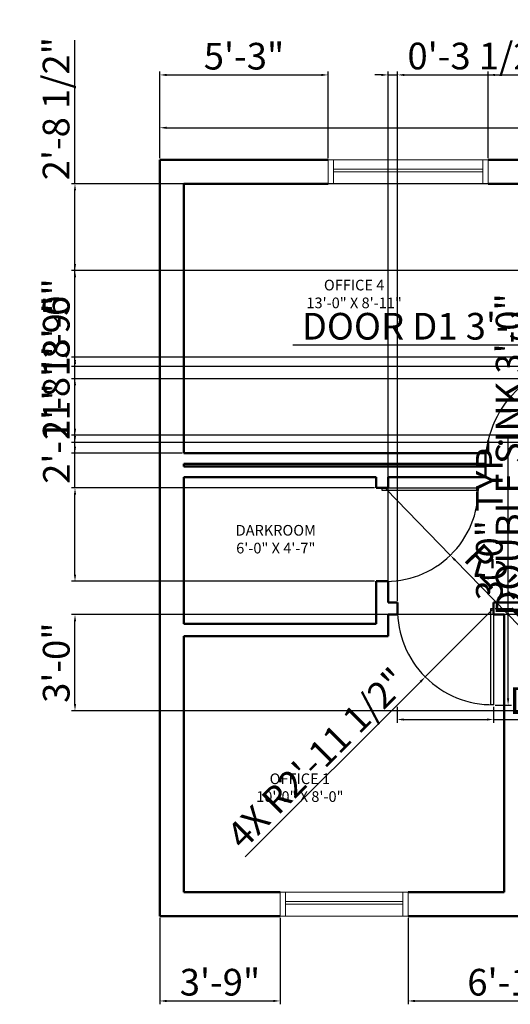
# Model space of a CAD drawing. Units: inches. Extents: x -53 to 650, y -41 to 348.
# Tile 1 of 3: x -53 to 131, y -33 to 336. Entities that reach past the tile are written whole.
import ezdxf

# ---------------------------------------------------------------- set-up
doc = ezdxf.new("R2010")
doc.units = ezdxf.units.IN
for name, color, linetype, lineweight in [('A-ANNO-DIMS', 2, 'Continuous', 18), ('A-AREA-IDEN', 7, 'Continuous', 25), ('A-DOOR', 3, 'Continuous', 25), ('A-GLAZ', 4, 'Continuous', 18), ('A-WALL', 7, 'Continuous', 50), ('A-WALL-PATT', 7, 'Continuous', 13)]:
    doc.layers.add(name, color=color, linetype=linetype, lineweight=lineweight)
doc.styles.get("Standard").update_dxf_attribs({"font": 'arial.ttf'})
doc.dimstyles.new('ISO-25', dxfattribs={"dimtxt": 10, "dimasz": 2.5, "dimexe": 1.25, "dimexo": 0.625, "dimtad": 1, "dimlunit": 4, "dimtxsty": 'Standard', "dimcen": 2.5, "dimadec": 0, "dimazin": 0, "dimtfac": 1, "dimtmove": 0, "dimatfit": 3, "dimfxl": 1, "dimarcsym": 0})

# ---------------------------------------------------------------- blocks, each defined once
blk = doc.blocks.new('*D4')
at = {"layer": 'A-ANNO-DIMS', "color": 0, "lineweight": -2, "transparency": 16777216}
for p, q in [((0, 284.12), (0, 296.76)), ((2.5, 295.51), (604.5, 295.51)), ((607, 284.12), (607, 296.76))]:
    blk.add_line(p, q, dxfattribs=at)
at = {"layer": 'A-ANNO-DIMS', "color": 0, "transparency": 16777216}
for points in [[(2.5, 295.92), (2.5, 295.09), (0, 295.51)], [(604.5, 295.92), (604.5, 295.09), (607, 295.51)]]:
    blk.add_solid(points, dxfattribs=at)
at = {"layer": 'Defpoints', "color": 0, "transparency": 16777216}
for p in [(607, 295.51), (0, 283.5), (607, 283.5)]:
    blk.add_point(p, dxfattribs=at)
at = {"layer": 'A-ANNO-DIMS', "color": 0, "transparency": 16777216, "insert": (303.5, 301.24), "char_height": 10, "attachment_point": 5}
blk.add_mtext('50\'-0"', dxfattribs=at)
blk = doc.blocks.new('DOOR-SWING-39IN')
for p, q in [((38, 0), (38, 39)), ((38, 39), (39, 39)), ((39, 39), (39, 0)), ((39, 0), (38, 0))]:
    blk.add_line(p, q)
blk.add_arc((38.5, 38.5), 38.5, 179.2559, 270.7441)
blk = doc.blocks.new('DOOR-SWING-36IN')
for p, q in [((35.001, 0.001), (35.001, 36.001)), ((35.001, 36.001), (36.001, 36.001)), ((36.001, 36.001), (36.001, 0.001)), ((36.001, 0.001), (35.001, 0.001))]:
    blk.add_line(p, q)
blk.add_arc((35.501, 35.501), 35.504, 179.19307, 270.80693)
blk = doc.blocks.new('WIN-48IN')
for p, q in [((0, 9), (0, 0)), ((2, 0), (2, 9)), ((46, 0), (46, 9)), ((48, 9), (48, 0)), ((2, 5.5), (46, 5.5)), ((2, 4.5), (46, 4.5))]:
    blk.add_line(p, q)
blk.add_lwpolyline([(48, 9), (0, 9), (0, 0), (48, 0)], close=True)
blk = doc.blocks.new('WIN-60IN')
for p, q in [((0, 9), (0, 0)), ((2, 0), (2, 9)), ((58, 0), (58, 9)), ((60, 9), (60, 0)), ((2, 5.5), (58, 5.5)), ((2, 4.5), (58, 4.5))]:
    blk.add_line(p, q)
blk.add_lwpolyline([(60, 9), (0, 9), (0, 0), (60, 0)], close=True)
blk = doc.blocks.new('*D11')
at = {"layer": 'A-ANNO-DIMS', "color": 0, "lineweight": -2, "transparency": 16777216}
for p, q in [((181.5, 208.76), (181.5, 215.26)), ((220.63, 208.76), (220.63, 215.26)), ((181.5, 214.01), (49.76, 214.01)), ((218.13, 214.01), (184, 214.01))]:
    blk.add_line(p, q, dxfattribs=at)
at = {"layer": 'A-ANNO-DIMS', "color": 0, "transparency": 16777216}
for points in [[(184, 214.42), (184, 213.59), (181.5, 214.01)], [(218.13, 214.42), (218.13, 213.59), (220.63, 214.01)]]:
    blk.add_solid(points, dxfattribs=at)
at = {"layer": 'Defpoints', "color": 0, "transparency": 16777216}
for p in [(181.5, 214.01), (181.5, 208.13), (220.63, 208.13)]:
    blk.add_point(p, dxfattribs=at)
at = {"layer": 'A-ANNO-DIMS', "color": 0, "transparency": 16777216, "insert": (114.38, 219.81), "char_height": 10, "attachment_point": 5}
blk.add_mtext('DOOR D1 3\'-3" TYP.', dxfattribs=at)
blk = doc.blocks.new('*D13')
at = {"layer": 'A-ANNO-DIMS', "color": 0, "lineweight": -2, "transparency": 16777216}
for p, q in [((88.86, 78.49), (88.86, 72.44)), ((125, 78.49), (125, 72.44)), ((91.36, 73.69), (122.5, 73.69)), ((125, 73.69), (256.74, 73.69))]:
    blk.add_line(p, q, dxfattribs=at)
at = {"layer": 'A-ANNO-DIMS', "color": 0, "transparency": 16777216}
for points in [[(91.36, 74.11), (91.36, 73.28), (88.86, 73.69)], [(122.5, 74.11), (122.5, 73.28), (125, 73.69)]]:
    blk.add_solid(points, dxfattribs=at)
at = {"layer": 'Defpoints', "color": 0, "transparency": 16777216}
for p in [(88.86, 79.11), (125, 79.11), (125, 73.69)]:
    blk.add_point(p, dxfattribs=at)
at = {"layer": 'A-ANNO-DIMS', "color": 0, "transparency": 16777216, "insert": (192.12, 79.5), "char_height": 10, "attachment_point": 5}
blk.add_mtext('DOOR D2 3\'-0" TYP.', dxfattribs=at)
blk = doc.blocks.new('*D14')
at = {"layer": 'A-ANNO-DIMS', "color": 0, "lineweight": -2, "transparency": 16777216}
for p, q in [((130.42, 115.25), (130.42, 179.95)), ((125.62, 115.25), (131.67, 115.25)), ((130.42, 81.61), (130.42, 112.75)), ((125.62, 79.11), (131.67, 79.11))]:
    blk.add_line(p, q, dxfattribs=at)
at = {"layer": 'A-ANNO-DIMS', "color": 0, "transparency": 16777216}
for points in [[(130, 112.75), (130.84, 112.75), (130.42, 115.25)], [(130, 81.61), (130.84, 81.61), (130.42, 79.11)]]:
    blk.add_solid(points, dxfattribs=at)
at = {"layer": 'Defpoints', "color": 0, "transparency": 16777216}
for p in [(125, 115.25), (130.42, 115.25), (125, 79.11)]:
    blk.add_point(p, dxfattribs=at)
at = {"layer": 'A-ANNO-DIMS', "color": 0, "transparency": 16777216, "insert": (124.69, 148.85), "char_height": 10, "attachment_point": 5, "rotation": 90}
blk.add_mtext('3\'-0" TYP.', dxfattribs=at)
blk = doc.blocks.new('*D21')
at = {"layer": 'A-ANNO-DIMS', "color": 0, "lineweight": -2, "transparency": 16777216}
for p, q in [((142.68, 274.14), (136.65, 274.14)), ((137.9, 271.64), (137.9, 240.64)), ((142.68, 238.14), (136.65, 238.14)), ((137.9, 238.14), (137.9, 110.49))]:
    blk.add_line(p, q, dxfattribs=at)
at = {"layer": 'A-ANNO-DIMS', "color": 0, "transparency": 16777216}
for points in [[(137.49, 271.64), (138.32, 271.64), (137.9, 274.14)], [(137.49, 240.64), (138.32, 240.64), (137.9, 238.14)]]:
    blk.add_solid(points, dxfattribs=at)
at = {"layer": 'Defpoints', "color": 0, "transparency": 16777216}
for p in [(143.3, 274.14), (137.9, 238.14), (143.3, 238.14)]:
    blk.add_point(p, dxfattribs=at)
at = {"layer": 'A-ANNO-DIMS', "color": 0, "transparency": 16777216, "insert": (132.1, 173.07), "char_height": 10, "attachment_point": 5, "rotation": 90}
blk.add_mtext('DOUBLE SINK 3\'-0"', dxfattribs=at)
blk = doc.blocks.new('*D27')
at = {"layer": 'A-ANNO-DIMS', "color": 0, "lineweight": -2, "transparency": 16777216}
for p, q in [((0, 284.12), (0, 316.56)), ((2.5, 315.31), (60.5, 315.31)), ((63, 284.12), (63, 316.56))]:
    blk.add_line(p, q, dxfattribs=at)
at = {"layer": 'A-ANNO-DIMS', "color": 0, "transparency": 16777216}
for points in [[(2.5, 315.72), (2.5, 314.89), (0, 315.31)], [(60.5, 315.72), (60.5, 314.89), (63, 315.31)]]:
    blk.add_solid(points, dxfattribs=at)
at = {"layer": 'Defpoints', "color": 0, "transparency": 16777216}
for p in [(63, 315.31), (0, 283.5), (63, 283.5)]:
    blk.add_point(p, dxfattribs=at)
at = {"layer": 'A-ANNO-DIMS', "color": 0, "transparency": 16777216, "insert": (31.5, 321.04), "char_height": 10, "attachment_point": 5}
blk.add_mtext('5\'-3"', dxfattribs=at)
blk = doc.blocks.new('*D28')
at = {"layer": 'A-ANNO-DIMS', "color": 0, "lineweight": -2, "transparency": 16777216}
for p, q in [((123, 284.12), (123, 316.56)), ((125.5, 315.31), (209, 315.31)), ((211.5, 284.12), (211.5, 316.56))]:
    blk.add_line(p, q, dxfattribs=at)
at = {"layer": 'A-ANNO-DIMS', "color": 0, "transparency": 16777216}
for points in [[(125.5, 315.72), (125.5, 314.89), (123, 315.31)], [(209, 315.72), (209, 314.89), (211.5, 315.31)]]:
    blk.add_solid(points, dxfattribs=at)
at = {"layer": 'Defpoints', "color": 0, "transparency": 16777216}
for p in [(211.5, 315.31), (123, 283.5), (211.5, 283.5)]:
    blk.add_point(p, dxfattribs=at)
at = {"layer": 'A-ANNO-DIMS', "color": 0, "transparency": 16777216, "insert": (167.25, 321.1), "char_height": 10, "attachment_point": 5}
blk.add_mtext('7\'-4 1/2"', dxfattribs=at)
blk = doc.blocks.new('*D32')
at = {"layer": 'A-ANNO-DIMS', "color": 0, "lineweight": -2, "transparency": 16777216}
for p, q in [((0, -0.62), (0, -33.05)), ((45, -0.62), (45, -33.05)), ((2.5, -31.8), (42.5, -31.8))]:
    blk.add_line(p, q, dxfattribs=at)
at = {"layer": 'A-ANNO-DIMS', "color": 0, "transparency": 16777216}
for points in [[(2.5, -31.39), (2.5, -32.22), (0, -31.8)], [(42.5, -31.39), (42.5, -32.22), (45, -31.8)]]:
    blk.add_solid(points, dxfattribs=at)
at = {"layer": 'Defpoints', "color": 0, "transparency": 16777216}
for p in [(0, 0), (45, 0), (45, -31.8)]:
    blk.add_point(p, dxfattribs=at)
at = {"layer": 'A-ANNO-DIMS', "color": 0, "transparency": 16777216, "insert": (22.5, -26.07), "char_height": 10, "attachment_point": 5}
blk.add_mtext('3\'-9"', dxfattribs=at)
blk = doc.blocks.new('*D33')
at = {"layer": 'A-ANNO-DIMS', "color": 0, "lineweight": -2, "transparency": 16777216}
for p, q in [((93, -0.62), (93, -33.05)), ((175, -0.62), (175, -33.05)), ((95.5, -31.8), (172.5, -31.8))]:
    blk.add_line(p, q, dxfattribs=at)
at = {"layer": 'A-ANNO-DIMS', "color": 0, "transparency": 16777216}
for points in [[(95.5, -31.39), (95.5, -32.22), (93, -31.8)], [(172.5, -31.39), (172.5, -32.22), (175, -31.8)]]:
    blk.add_solid(points, dxfattribs=at)
at = {"layer": 'Defpoints', "color": 0, "transparency": 16777216}
for p in [(93, 0), (175, 0), (175, -31.8)]:
    blk.add_point(p, dxfattribs=at)
at = {"layer": 'A-ANNO-DIMS', "color": 0, "transparency": 16777216, "insert": (134, -26.07), "char_height": 10, "attachment_point": 5}
blk.add_mtext('6\'-10"', dxfattribs=at)
blk = doc.blocks.new('*D39')
at = {"layer": 'A-ANNO-DIMS', "color": 0, "lineweight": -2, "transparency": 16777216}
for p, q in [((312.88, 242), (-33.06, 242)), ((-31.81, 208.5), (-31.81, 239.5)), ((312.88, 206), (-33.06, 206))]:
    blk.add_line(p, q, dxfattribs=at)
at = {"layer": 'A-ANNO-DIMS', "color": 0, "transparency": 16777216}
for points in [[(-32.22, 239.5), (-31.39, 239.5), (-31.81, 242)], [(-32.22, 208.5), (-31.39, 208.5), (-31.81, 206)]]:
    blk.add_solid(points, dxfattribs=at)
at = {"layer": 'Defpoints', "color": 0, "transparency": 16777216}
for p in [(-31.81, 242), (313.5, 242), (313.5, 206)]:
    blk.add_point(p, dxfattribs=at)
at = {"layer": 'A-ANNO-DIMS', "color": 0, "transparency": 16777216, "insert": (-37.54, 224), "char_height": 10, "attachment_point": 5, "rotation": 90}
blk.add_mtext('3\'-0"', dxfattribs=at)
blk = doc.blocks.new('*D40')
at = {"layer": 'A-ANNO-DIMS', "color": 0, "lineweight": -2, "transparency": 16777216}
for p, q in [((-31.81, 274.5), (-31.81, 328.3)), ((312.88, 274.5), (-33.06, 274.5)), ((-31.81, 244.5), (-31.81, 272)), ((312.88, 242), (-33.06, 242))]:
    blk.add_line(p, q, dxfattribs=at)
at = {"layer": 'A-ANNO-DIMS', "color": 0, "transparency": 16777216}
for points in [[(-32.22, 272), (-31.39, 272), (-31.81, 274.5)], [(-32.22, 244.5), (-31.39, 244.5), (-31.81, 242)]]:
    blk.add_solid(points, dxfattribs=at)
at = {"layer": 'Defpoints', "color": 0, "transparency": 16777216}
for p in [(-31.81, 274.5), (313.5, 274.5), (313.5, 242)]:
    blk.add_point(p, dxfattribs=at)
at = {"layer": 'A-ANNO-DIMS', "color": 0, "transparency": 16777216, "insert": (-37.6, 302.65), "char_height": 10, "attachment_point": 5, "rotation": 90}
blk.add_mtext('2\'-8 1/2"', dxfattribs=at)
blk = doc.blocks.new('*D43')
at = {"layer": 'A-ANNO-DIMS', "color": 0, "lineweight": -2, "transparency": 16777216}
for p, q in [((505.38, 113), (-33.05, 113)), ((-31.81, 79.5), (-31.81, 110.5)), ((505.38, 77), (-33.05, 77))]:
    blk.add_line(p, q, dxfattribs=at)
at = {"layer": 'A-ANNO-DIMS', "color": 0, "transparency": 16777216}
for points in [[(-32.22, 110.5), (-31.39, 110.5), (-31.81, 113)], [(-32.22, 79.5), (-31.39, 79.5), (-31.81, 77)]]:
    blk.add_solid(points, dxfattribs=at)
at = {"layer": 'Defpoints', "color": 0, "transparency": 16777216}
for p in [(-31.81, 113), (506, 113), (506, 77)]:
    blk.add_point(p, dxfattribs=at)
at = {"layer": 'A-ANNO-DIMS', "color": 0, "transparency": 16777216, "insert": (-37.54, 95), "char_height": 10, "attachment_point": 5, "rotation": 90}
blk.add_mtext('3\'-0"', dxfattribs=at)
blk = doc.blocks.new('*D48')
at = {"layer": 'A-ANNO-DIMS', "color": 0, "lineweight": -2, "transparency": 16777216}
for p, q in [((83, 315.31), (80.5, 315.31)), ((85.5, 118.12), (85.5, 316.56)), ((85.5, 315.31), (89, 315.31)), ((89, 118.12), (89, 316.56)), ((91.5, 315.31), (145.13, 315.31))]:
    blk.add_line(p, q, dxfattribs=at)
at = {"layer": 'A-ANNO-DIMS', "color": 0, "transparency": 16777216}
for points in [[(83, 315.72), (83, 314.89), (85.5, 315.31)], [(91.5, 315.72), (91.5, 314.89), (89, 315.31)]]:
    blk.add_solid(points, dxfattribs=at)
at = {"layer": 'Defpoints', "color": 0, "transparency": 16777216}
for p in [(89, 315.31), (85.5, 117.5), (89, 117.5)]:
    blk.add_point(p, dxfattribs=at)
at = {"layer": 'A-ANNO-DIMS', "color": 0, "transparency": 16777216, "insert": (119.57, 321.1), "char_height": 10, "attachment_point": 5}
blk.add_mtext('0\'-3 1/2"', dxfattribs=at)
blk = doc.blocks.new('*D51')
at = {"layer": 'A-ANNO-DIMS', "color": 0, "lineweight": -2, "transparency": 16777216}
for p, q in [((-31.81, 160.5), (-31.81, 198.77)), ((80.38, 160.5), (-33.06, 160.5)), ((-31.81, 128), (-31.81, 158)), ((80.38, 125.5), (-33.06, 125.5))]:
    blk.add_line(p, q, dxfattribs=at)
at = {"layer": 'A-ANNO-DIMS', "color": 0, "transparency": 16777216}
for points in [[(-32.22, 158), (-31.39, 158), (-31.81, 160.5)], [(-32.22, 128), (-31.39, 128), (-31.81, 125.5)]]:
    blk.add_solid(points, dxfattribs=at)
at = {"layer": 'Defpoints', "color": 0, "transparency": 16777216}
for p in [(-31.81, 160.5), (81, 160.5), (81, 125.5)]:
    blk.add_point(p, dxfattribs=at)
at = {"layer": 'A-ANNO-DIMS', "color": 0, "transparency": 16777216, "insert": (-37.45, 180.89), "char_height": 10, "attachment_point": 5, "rotation": 90}
blk.add_mtext('2\'-11"', dxfattribs=at)
blk = doc.blocks.new('*D52')
at = {"layer": 'A-ANNO-DIMS', "color": 0, "lineweight": -2, "transparency": 16777216}
for p, q in [((562.88, 209.5), (-33.06, 209.5)), ((-31.81, 180), (-31.81, 207)), ((562.88, 177.5), (-33.06, 177.5))]:
    blk.add_line(p, q, dxfattribs=at)
at = {"layer": 'A-ANNO-DIMS', "color": 0, "transparency": 16777216}
for points in [[(-32.22, 207), (-31.39, 207), (-31.81, 209.5)], [(-32.22, 180), (-31.39, 180), (-31.81, 177.5)]]:
    blk.add_solid(points, dxfattribs=at)
at = {"layer": 'Defpoints', "color": 0, "transparency": 16777216}
for p in [(-31.81, 209.5), (563.5, 209.5), (563.5, 177.5)]:
    blk.add_point(p, dxfattribs=at)
at = {"layer": 'A-ANNO-DIMS', "color": 0, "transparency": 16777216, "insert": (-37.54, 193.5), "char_height": 10, "attachment_point": 5, "rotation": 90}
blk.add_mtext('2\'-8"', dxfattribs=at)
blk = doc.blocks.new('*D54')
at = {"layer": 'A-ANNO-DIMS', "color": 0, "lineweight": -2, "transparency": 16777216}
for p, q in [((8.38, 274.5), (-33.06, 274.5)), ((-31.81, 176), (-31.81, 272)), ((8.38, 173.5), (-33.06, 173.5))]:
    blk.add_line(p, q, dxfattribs=at)
at = {"layer": 'A-ANNO-DIMS', "color": 0, "transparency": 16777216}
for points in [[(-32.22, 272), (-31.39, 272), (-31.81, 274.5)], [(-32.22, 176), (-31.39, 176), (-31.81, 173.5)]]:
    blk.add_solid(points, dxfattribs=at)
at = {"layer": 'Defpoints', "color": 0, "transparency": 16777216}
for p in [(-31.81, 274.5), (9, 274.5), (9, 173.5)]:
    blk.add_point(p, dxfattribs=at)
at = {"layer": 'A-ANNO-DIMS', "color": 0, "transparency": 16777216, "insert": (-37.54, 224), "char_height": 10, "attachment_point": 5, "rotation": 90}
blk.add_mtext('8\'-5"', dxfattribs=at)
blk = doc.blocks.new('*D56')
at = {"layer": 'A-ANNO-DIMS', "color": 0, "lineweight": -2, "transparency": 16777216}
for p, q in [((-31.81, 201.42), (-31.81, 230.81)), ((570.47, 201.42), (-33.05, 201.42)), ((-31.81, 182.73), (-31.81, 198.92)), ((570.47, 180.23), (-33.05, 180.23))]:
    blk.add_line(p, q, dxfattribs=at)
at = {"layer": 'A-ANNO-DIMS', "color": 0, "transparency": 16777216}
for points in [[(-32.22, 198.92), (-31.39, 198.92), (-31.81, 201.42)], [(-32.22, 182.73), (-31.39, 182.73), (-31.81, 180.23)]]:
    blk.add_solid(points, dxfattribs=at)
at = {"layer": 'Defpoints', "color": 0, "transparency": 16777216}
for p in [(-31.81, 201.42), (571.1, 201.42), (571.1, 180.23)]:
    blk.add_point(p, dxfattribs=at)
at = {"layer": 'A-ANNO-DIMS', "color": 0, "transparency": 16777216, "insert": (-37.54, 217.37), "char_height": 10, "attachment_point": 5, "rotation": 90}
blk.add_mtext('1\'-9"', dxfattribs=at)
blk = doc.blocks.new('*D60')
at = {"layer": 'A-ANNO-DIMS', "color": 0, "lineweight": -2, "transparency": 16777216}
for p, q in [((84.72, 160), (108.79, 135.24)), ((160.01, 82.56), (110.54, 133.45))]:
    blk.add_line(p, q, dxfattribs=at)
at = {"layer": 'A-ANNO-DIMS', "color": 0, "transparency": 16777216}
blk.add_solid([(110.83, 133.74), (110.24, 133.16), (108.79, 135.24)], dxfattribs=at)
at = {"layer": 'Defpoints', "color": 0, "transparency": 16777216}
for p in [(84.72, 160), (108.79, 135.24)]:
    blk.add_point(p, dxfattribs=at)
at = {"layer": 'A-ANNO-DIMS', "color": 0, "transparency": 16777216, "insert": (140.3, 111.15), "char_height": 10, "attachment_point": 5, "rotation": 314.1925}
blk.add_mtext('R2\'-10 1/2"', dxfattribs=at)
blk = doc.blocks.new('*D63')
at = {"layer": 'A-ANNO-DIMS', "color": 0, "lineweight": -2, "transparency": 16777216}
for p, q in [((124.5, 114.75), (99.4, 89.65)), ((31.96, 22.21), (97.63, 87.88))]:
    blk.add_line(p, q, dxfattribs=at)
at = {"layer": 'A-ANNO-DIMS', "color": 0, "transparency": 16777216}
blk.add_solid([(97.33, 88.17), (97.92, 87.58), (99.4, 89.65)], dxfattribs=at)
at = {"layer": 'Defpoints', "color": 0, "transparency": 16777216}
for p in [(124.5, 114.75), (99.4, 89.65)]:
    blk.add_point(p, dxfattribs=at)
at = {"layer": 'A-ANNO-DIMS', "color": 0, "transparency": 16777216, "insert": (59.81, 58.26), "char_height": 10, "attachment_point": 5, "rotation": 45}
blk.add_mtext('4X R2\'-11 1/2"', dxfattribs=at)

msp = doc.modelspace()

# ---------------------------------------------------------------- hatches: boundary and pattern name
at = {"layer": 'A-WALL-PATT'}
h = msp.add_hatch(color=256, dxfattribs=at)
h.dxf.hatch_style = 1
h.paths.add_polyline_path([(9, 169.5), (9, 168.5), (122, 168.5), (122, 169, -0.0032466), (121.997, 169.5)])
h.paths.add_polyline_path([(161, 169.5), (161, 168.5), (181.5, 168.5), (181.5, 169.5)])
h.paths.add_polyline_path([(220.503, 169.5), (220.503, 168.5), (390, 168.5), (390, 169.5)])
h.paths.add_polyline_path([(598, 168.5), (598, 169.5), (438, 169.5), (438, 168.5)])

# ---------------------------------------------------------------- linework, layer by layer
at = {"layer": 'A-DOOR'}
for p, q in [((83.25, 160.5), (119.25, 160.5)), ((83.25, 159.5), (83.25, 160.5)), ((119.25, 159.5), (83.25, 159.5)), ((119.25, 160.5), (119.25, 159.5))]:
    msp.add_line(p, q, dxfattribs=at)
msp.add_arc((84.722, 160), 34.531, 267.55649, 0.82965, dxfattribs=at)
at = {"layer": 'A-WALL'}
for p, q in [((0, 283.5), (63, 283.5)), ((0, 283.5), (0, 0)), ((123, 283.5), (467.5, 283.5)), ((9, 274.5), (9, 173.5)), ((9, 274.5), (63, 274.5)), ((123, 274.5), (165, 274.5)), ((123, 178.232), (123, 173.5)), ((9, 173.5), (122, 173.5)), ((122, 173.5), (122, 164.5)), ((9, 169.5), (122, 169.5)), ((9, 169.5), (9, 168.5)), ((9, 168.5), (122, 168.5)), ((122, 169.5), (122, 168.5)), ((9, 164.5), (81, 164.5)), ((9, 164.5), (9, 109.5)), ((81, 164.5), (81, 160.5)), ((85.5, 164.5), (85.5, 160.5)), ((85.5, 164.5), (122, 164.5)), ((81, 160.5), (85.5, 160.5)), ((81, 125.5), (81, 109.5)), ((81, 125.5), (85.5, 125.5)), ((85.5, 125.5), (85.5, 117.5)), ((85.5, 117.5), (89, 117.5)), ((89, 117.5), (89, 113)), ((125, 117.5), (125, 113)), ((125, 117.5), (219.5, 117.5)), ((85.5, 113), (89, 113)), ((85.5, 113), (85.5, 105)), ((125, 113), (129, 113)), ((129, 113), (129, 9)), ((9, 109.5), (81, 109.5)), ((9, 105), (85.5, 105)), ((9, 105), (9, 9)), ((9, 9), (45, 9)), ((93, 9), (129, 9)), ((0, 0), (45, 0)), ((93, 0), (607, 0))]:
    msp.add_line(p, q, dxfattribs=at)

# ---------------------------------------------------------------- block references
at = {"layer": 'A-DOOR', "extrusion": (0, 0, -1), "zscale": -1, "rotation": 180}
msp.add_blockref('DOOR-SWING-39IN', (-122, 208), dxfattribs=at)
at = {"layer": 'A-DOOR'}
msp.add_blockref('DOOR-SWING-36IN', (88.999, 79.249), dxfattribs=at)
at = {"layer": 'A-GLAZ'}
for name, p in [('WIN-60IN', (63, 274.5)), ('WIN-48IN', (45, 0))]:
    msp.add_blockref(name, p, dxfattribs=at)

# ---------------------------------------------------------------- texts
at = {"layer": 'A-AREA-IDEN', "char_height": 4, "attachment_point": 1}
for s, insert in [('\\pxqc;OFFICE 4\\P13\'-0" X 8\'-11"', (39.982, 238.539)), ('\\pxqc;DARKROOM\\P6\'-0" X 4\'-7"', (10.647, 146.62)), ('\\pxqc;OFFICE 1\\P10\'-0" X 8\'-0"', (19.651, 53.482))]:
    msp.add_mtext_dynamic_manual_height_columns(s, width=65.53067, gutter_width=12.5, heights=[0], dxfattribs=dict(at, insert=insert))

# ---------------------------------------------------------------- dimensions: what is measured, and where the dimension line sits
at = {"layer": 'A-ANNO-DIMS'}
for base, p1, p2, picture, middle in [((89, 315.305), (85.5, 117.5), (89, 117.5), '*D48', (119.567, 321.104)), ((211.5, 315.305), (123, 283.5), (211.5, 283.5), '*D28', (167.25, 321.101)), ((63, 315.305), (0, 283.5), (63, 283.5), '*D27', (31.5, 321.039)), ((45, -31.805), (0, 0), (45, 0), '*D32', (22.5, -26.071)), ((175, -31.805), (93, 0), (175, 0), '*D33', (134, -26.074))]:
    dim = msp.add_linear_dim(base=base, p1=p1, p2=p2, dimstyle='ISO-25', override={"dimdec": 1, "dimlfac": 1, "dimrnd": 0, "dimzin": 1, "dimdsep": 46, "dimlunit": 4, "dimfrac": 2}, dxfattribs=at)
    dim.commit()
    dim.dimension.update_dxf_attribs({"geometry": picture, "text_midpoint": middle})
for base, p1, p2, picture, middle in [((-31.805, 274.5), (313.5, 242), (313.5, 274.5), '*D40', (-37.601, 302.652)), ((-31.805, 274.5), (9, 173.5), (9, 274.5), '*D54', (-37.536, 224)), ((-31.805, 242), (313.5, 206), (313.5, 242), '*D39', (-37.539, 224)), ((-31.805, 201.421), (571.095, 180.228), (571.095, 201.421), '*D56', (-37.536, 217.367)), ((-31.805, 209.5), (563.5, 177.5), (563.5, 209.5), '*D52', (-37.536, 193.5)), ((-31.805, 160.5), (81, 125.5), (81, 160.5), '*D51', (-37.45, 180.886)), ((-31.805, 113), (506, 77), (506, 113), '*D43', (-37.539, 95))]:
    dim = msp.add_linear_dim(base=base, p1=p1, p2=p2, angle=90, dimstyle='ISO-25', override={"dimdec": 1, "dimlfac": 1, "dimrnd": 0, "dimzin": 1, "dimdsep": 46, "dimlunit": 4, "dimfrac": 2}, dxfattribs=at)
    dim.commit()
    dim.dimension.update_dxf_attribs({"geometry": picture, "text_midpoint": middle})
for base, p1, p2, text, override, picture, middle in [((607, 295.508), (0, 283.5), (607, 283.5), '50\'-0"', {"dimclrd": 0, "dimclre": 0, "dimclrt": 0}, '*D4', (303.5, 301.239)), ((125, 73.695), (88.865, 79.115), (125, 79.115), 'DOOR D2 <> TYP.', {"dimdec": 1, "dimlfac": 1, "dimrnd": 0, "dimzin": 1, "dimdsep": 46, "dimlunit": 4, "dimfrac": 2}, '*D13', (192.119, 79.497))]:
    dim = msp.add_linear_dim(base=base, p1=p1, p2=p2, text=text, dimstyle='ISO-25', override=override, dxfattribs=at)
    dim.commit()
    dim.dimension.update_dxf_attribs({"geometry": picture, "text_midpoint": middle})
for base, p1, p2, angle, text, picture, middle in [((137.904, 238.142), (143.304, 274.142), (143.304, 238.142), 270, 'DOUBLE SINK <>', '*D21', (132.102, 173.066)), ((181.5, 214.005), (220.635, 208.135), (181.5, 208.135), 180, 'DOOR D1 <> TYP.', '*D11', (114.381, 219.807)), ((130.42, 115.25), (125, 79.115), (125, 115.25), 90, '<> TYP.', '*D14', (124.686, 148.849))]:
    dim = msp.add_linear_dim(base=base, p1=p1, p2=p2, angle=angle, text=text, dimstyle='ISO-25', override={"dimdec": 1, "dimlfac": 1, "dimrnd": 0, "dimzin": 1, "dimdsep": 46, "dimlunit": 4, "dimfrac": 2}, dxfattribs=at)
    dim.commit()
    dim.dimension.update_dxf_attribs({"geometry": picture, "text_midpoint": middle})
dim = msp.add_radius_dim(center=(84.722, 160), mpoint=(108.793, 135.241), dimstyle='ISO-25', override={"dimdec": 1, "dimlfac": 1, "dimrnd": 0, "dimzin": 1, "dimdsep": 46, "dimlunit": 4, "dimfrac": 2}, dxfattribs=at)
dim.commit()
dim.dimension.update_dxf_attribs({"geometry": '*D60', "text_midpoint": (140.299, 111.148)})
dim = msp.add_radius_dim(center=(124.5, 114.75), mpoint=(99.395, 89.645), text='4X <>', dimstyle='ISO-25', override={"dimdec": 1, "dimlfac": 1, "dimrnd": 0, "dimzin": 1, "dimdsep": 46, "dimlunit": 4, "dimfrac": 2}, dxfattribs=at)
dim.commit()
dim.dimension.update_dxf_attribs({"geometry": '*D63', "text_midpoint": (59.813, 58.26)})

doc.saveas('drawing.dxf')
